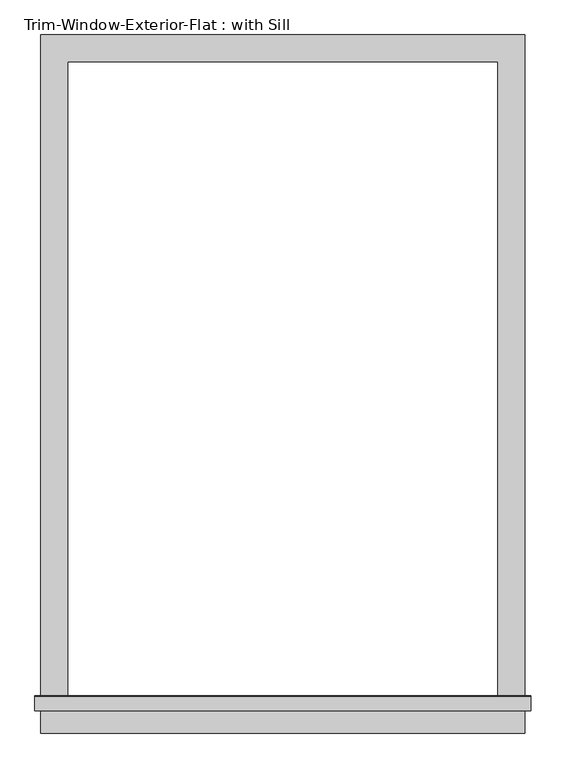
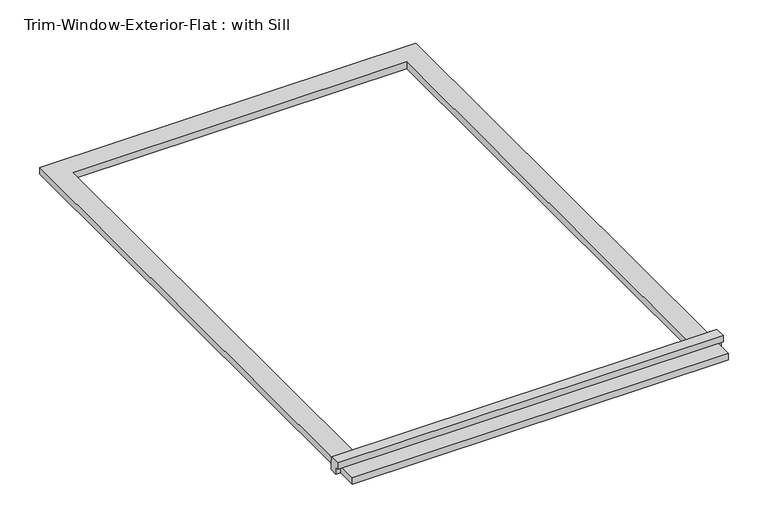
"""IFC4 building model written with IfcOpenShell, lengths in millimetres: proxy geometry, Trim-Window-Exterior-Flat : with Sill."""

from ifc_helpers import new_model, si_unit, frame, origin, origin_with_axes, place, context, project, spatial, polyline, outline, extrude, source, transform, mapped, element, save


def trim_window_exterior_flat_with_sill_66148908(model_context):
    return source(origin(), model_context, "Body", "SweptSolid", [
        extrude(outline(polyline([(514.35, -1368.3823709), (514.35, -1425.5323709), (-514.35, -1425.5323709), (-514.35, -1368.3823709), (514.35, -1368.3823709)])), origin_with_axes(), (0.0, 0.0, 1.0), 19.05),
        extrude(outline(polyline([(-1377.95, 38.1), (-1348.6580645, 38.1), (-1346.2, 19.05), (-1346.2, 0.0), (-1368.3823709, 0.0), (-1368.3823709, 19.05), (-1377.95, 19.05), (-1377.95, 38.1)])), frame((-527.05, 0.0, 0.0), z_axis=(1.0, 0.0, 0.0), x_axis=(0.0, 1.0, 0.0)), (0.0, 0.0, 1.0), 1054.1),
        extrude(outline(polyline([(-514.35, 57.15), (514.35, 57.15), (514.35, -1346.2), (457.2, -1346.2), (457.2, 0.0), (-457.2, 0.0), (-457.2, -1346.2), (-514.35, -1346.2), (-514.35, 57.15)])), origin_with_axes(), (0.0, 0.0, 1.0), 19.05),
    ])


if __name__ == "__main__":
    model = new_model("IFC4")
    model_context = context("Model", 3, world=origin())
    ifc_project = project(units=[si_unit("LENGTHUNIT", "METRE", prefix="MILLI")], contexts=[model_context])
    site = spatial("IfcSite", under=ifc_project)
    building = spatial("IfcBuilding", under=site)
    placement = place(None, origin())
    trim_window_exterior_flat_with_sill_shape = trim_window_exterior_flat_with_sill_66148908(model_context)
    element("IfcBuildingElementProxy", 1, Name="Trim-Window-Exterior-Flat : with Sill", ObjectType="Trim-Window-Exterior-Flat : with Sill", at=placement, inside=building, context=model_context, shape_type="MappedRepresentation", body=[
        mapped(trim_window_exterior_flat_with_sill_shape, transform((0.0, 0.0, 0.0), x_axis=(1.0, 0.0, 0.0), y_axis=(0.0, 1.0, 0.0), z_axis=(0.0, 0.0, 1.0))),
    ])
    save(model, "model.ifc")

# Revit data of these elements
# Type "Trim-Window-Exterior-Flat : with Sill"
#   Trim Width = 0' - 2 1/4"
#   Trim Thickness_Picture Frame = 0' - 1 1/4"
#   Trim Thickness_with Sill = 0' - 0 3/4"
#   Sill Thickness = 0' - 1 1/4"
#   Opening Width [instance default] = 2' - 0"
#   Opening Height [instance default] = 3' - 0"
#   Default Elevation = 4' - 0"
#   Sill = yes
#   Picture Frame = no
#   Trim Material [instance default] = none
# Element 1 (IfcBuildingElementProxy, "Trim-Window-Exterior-Flat : with Sill")
#   Opening Width = 3' - 0"
#   Opening Height = 4' - 5"
#   Trim Material = Clad - White
#   Materials on its faces: "Clad - White"
# Materials
#   "Clad - White": class "Wood", colour RGB 242 242 238, transparency 0, Cost = 0
